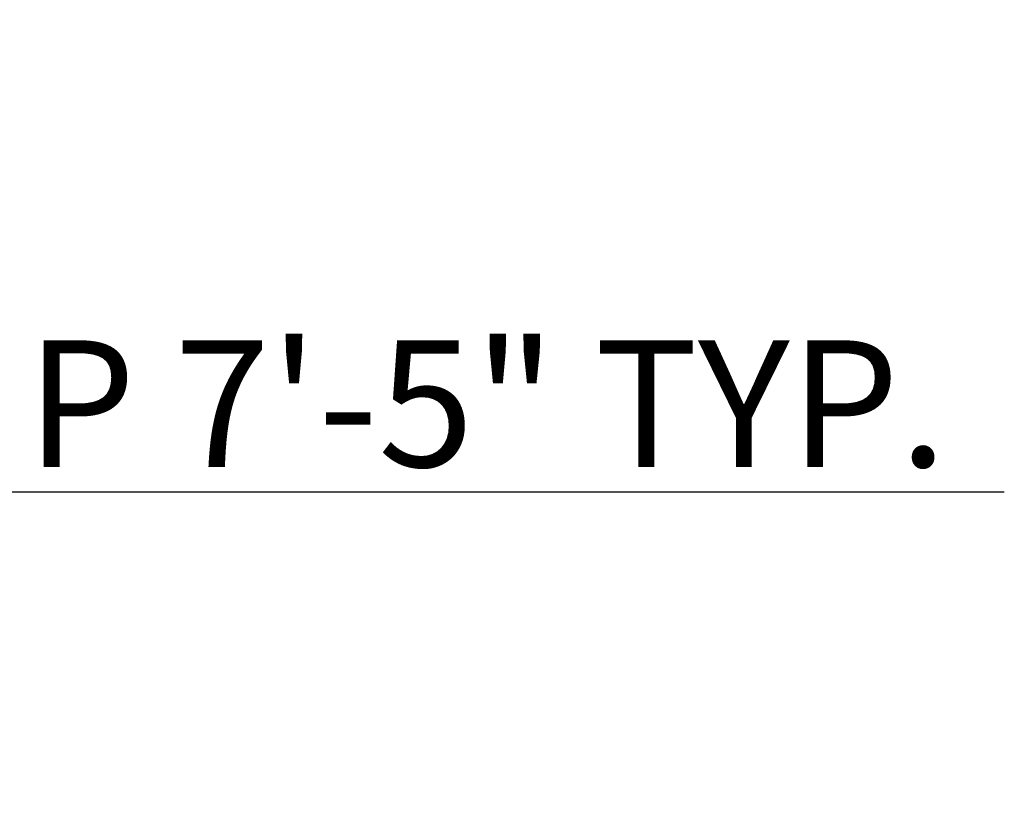
# Model space of a CAD drawing. Units: inches. Extents: x 1763 to 2368, y 1500 to 2097.
# Tile 24 of 24: x 2271 to 2368, y 1930 to 2009. Entities that reach past the tile are written whole.
import ezdxf

# ---------------------------------------------------------------- set-up
doc = ezdxf.new("R2010")
doc.units = ezdxf.units.IN
doc.layers.add('A-ANNO-DIMS', color=2, linetype='Continuous', lineweight=18)
doc.styles.get("Standard").update_dxf_attribs({"font": 'arial.ttf'})
doc.dimstyles.new('ISO-25', dxfattribs={"dimtxt": 12.5, "dimasz": 2.5, "dimexe": 1.25, "dimexo": 0.625, "dimtad": 1, "dimdec": 0, "dimlunit": 4, "dimtxsty": 'Standard', "dimblk": 'ARCHTICK', "dimcen": 2.5, "dimclrd": 3, "dimclrt": 4, "dimadec": 0, "dimazin": 0, "dimtfac": 1, "dimtdec": 0, "dimtmove": 0, "dimatfit": 3, "dimfxl": 1, "dimarcsym": 0})

# ---------------------------------------------------------------- blocks, each defined once
blk = doc.blocks.new('_ArchTick')
at = {"color": 0, "linetype": 'ByBlock', "const_width": 0.15}
blk.add_lwpolyline([(-0.5, -0.5), (0.5, 0.5)], dxfattribs=at)
blk = doc.blocks.new('*D23')
at = {"layer": 'A-ANNO-DIMS', "color": 0, "lineweight": -2, "transparency": 16777216}
for p, q in [((2089.477, 1949.977), (2089.477, 1963.985)), ((2178.698, 1949.977), (2178.698, 1963.985))]:
    blk.add_line(p, q, dxfattribs=at)
at = {"layer": 'A-ANNO-DIMS', "color": 3, "lineweight": -2, "transparency": 16777216}
for p, q in [((2089.477, 1962.735), (2178.698, 1962.735)), ((2178.698, 1962.735), (2367.732, 1962.735))]:
    blk.add_line(p, q, dxfattribs=at)
at = {"layer": 'Defpoints', "color": 0, "transparency": 16777216}
for p in [(2178.698, 1962.735), (2089.477, 1949.352), (2178.698, 1949.352)]:
    blk.add_point(p, dxfattribs=at)
at = {"layer": 'A-ANNO-DIMS', "color": 3, "lineweight": -2, "transparency": 16777216, "xscale": 2.5, "yscale": 2.5, "zscale": 2.5, "rotation": 180}
blk.add_blockref('_ArchTick', (2089.477, 1962.735), dxfattribs=at)
at = {"layer": 'A-ANNO-DIMS', "color": 3, "lineweight": -2, "transparency": 16777216, "xscale": 2.5, "yscale": 2.5, "zscale": 2.5}
blk.add_blockref('_ArchTick', (2178.698, 1962.735), dxfattribs=at)
at = {"layer": 'A-ANNO-DIMS', "color": 4, "transparency": 16777216, "insert": (2274.465, 1969.828), "char_height": 12.5, "attachment_point": 5}
blk.add_mtext('BED GROUP 7\'-5" TYP.', dxfattribs=at)

msp = doc.modelspace()

# ---------------------------------------------------------------- dimensions: what is measured, and where the dimension line sits
at = {"layer": 'A-ANNO-DIMS'}
dim = msp.add_linear_dim(base=(2178.698, 1962.735), p1=(2089.477, 1949.352), p2=(2178.698, 1949.352), text='BED GROUP <> TYP.', dimstyle='ISO-25', override={"dimdec": 1, "dimlfac": 1, "dimrnd": 0, "dimzin": 1, "dimdsep": 46, "dimlunit": 4, "dimfrac": 2}, dxfattribs=at)
dim.commit()
dim.dimension.update_dxf_attribs({"geometry": '*D23', "text_midpoint": (2274.465, 1969.828)})

doc.saveas('drawing.dxf')
